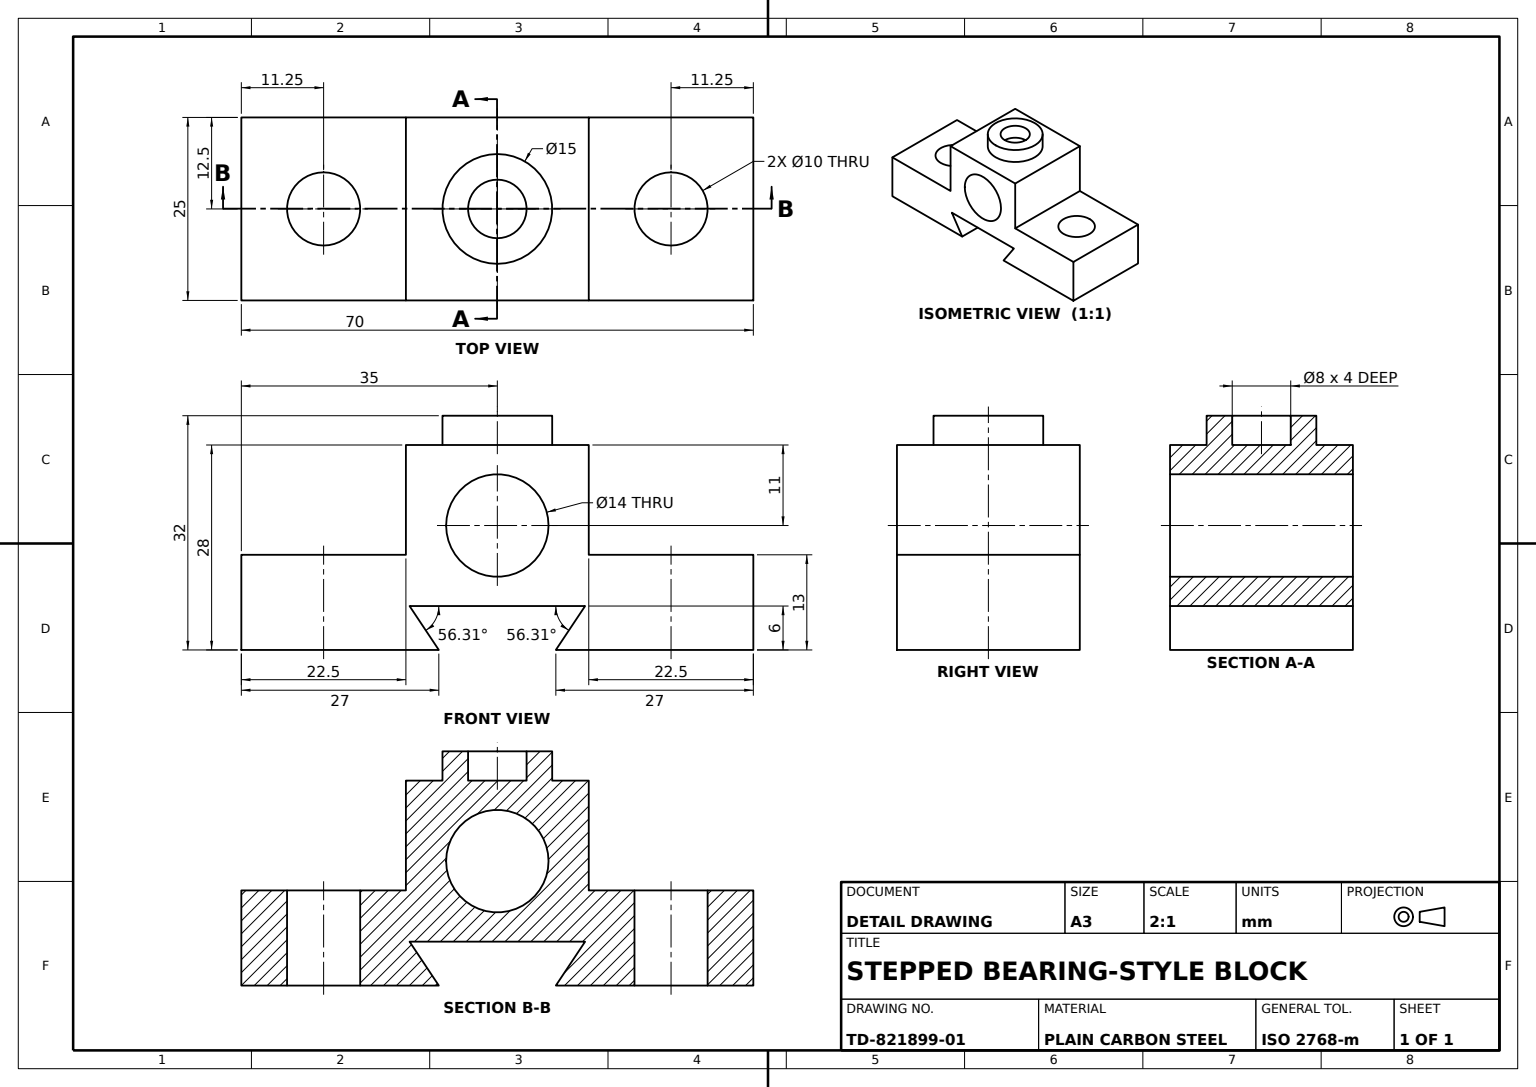
SolidWorks part; units mm, degrees
material "Plain Carbon Steel"
ref_plane "Front Plane" through (0, 0, 0) normal (0, 0, 1) x (1, 0, 0)
ref_plane "Top Plane" through (0, 0, 0) normal (0, 1, 0) x (1, 0, 0)
ref_plane "Right Plane" through (0, 0, 0) normal (1, 0, 0) x (0, 0, -1)
sketch "Stepped Block Profile" plane through (0, 0, 0) normal (0, 0, 1) x (1, 0, 0)
  line L0 (0, 0) -> (0, 13)
  line L1 (0, 0) -> (27, 0)
  line L2 (70, 0) -> (70, 13)
  line L3 (27, 0) -> (23, 6)
  line L4 (35, 6) -> (47, 6)
  line L5 (35, 6) -> (23, 6)
  line L6 (70, 0) -> (43, 0)
  line L7 (43, 0) -> (47, 6)
  line L9 (35, 28) -> (47.5, 28)
  line L10 (47.5, 28) -> (47.5, 13)
  line L11 (47.5, 13) -> (70, 13)
  line L12 (35, 28) -> (22.5, 28)
  line L13 (22.5, 28) -> (22.5, 13)
  line L14 (22.5, 13) -> (0, 13)
  dimension "D1" = 70
  dimension "D2" = 22.5
  dimension "D3" = 23
  dimension "D4" = 27
  dimension "D5" = 6
  dimension "D6" = 13
  dimension "D7" = 28
extrude "Stepped Block" add sketch "Stepped Block Profile" along normal blind 25
sketch "Cross Hole Sketch" plane through (0, 0, 25) normal (0, 0, 1) x (1, 0, 0)
  line L0 (47.5, 28) -> (22.5, 28) construction
  line L1 (70, 0) -> (70, 13) construction
  circle A0 centre (35, 17) radius 7
  dimension "D1" = 11
  dimension "D2" = 14
  dimension "D3" = 35
extrude "Cross Hole Ø11" cut sketch "Cross Hole Sketch" against normal blind 25
sketch "Step Holes Sketch" plane through (0, 13, 0) normal (0, 1, 0) x (1, 0, 0)
  line L0 (47.5, -25) -> (47.5, 0) construction
  line L1 (70, 0) -> (47.5, 0) construction
  circle A0 centre (58.75, -12.5) radius 5
  circle A1 centre (11.25, -12.5) radius 5
  dimension "D1" = 10
  dimension "D2" = 11.25
  dimension "D3" = 36.25
  dimension "D4" = 12.5
extrude "Step Holes 2x Depth 13" cut sketch "Step Holes Sketch" against normal blind 13
sketch "Top Boss Sketch" plane through (0, 28, 0) normal (0, 1, 0) x (1, 0, 0)
  line L0 (22.5, -25) -> (22.5, 0) construction
  line L1 (47.5, 0) -> (22.5, 0) construction
  circle A0 centre (35, -12.5) radius 7.5
  dimension "D1" = 15
  dimension "D2" = 12.5
  dimension "D3" = 12.5
extrude "Top Boss" add sketch "Top Boss Sketch" along normal blind 4
sketch "Top Boss Bore Sketch" plane through (0, 32, 0) normal (0, 1, 0) x (1, 0, 0)
  circle A0 centre (35, -12.5) radius 4
  dimension "D1" = 8
extrude "Top Boss Bore" cut sketch "Top Boss Bore Sketch" against normal blind 4
